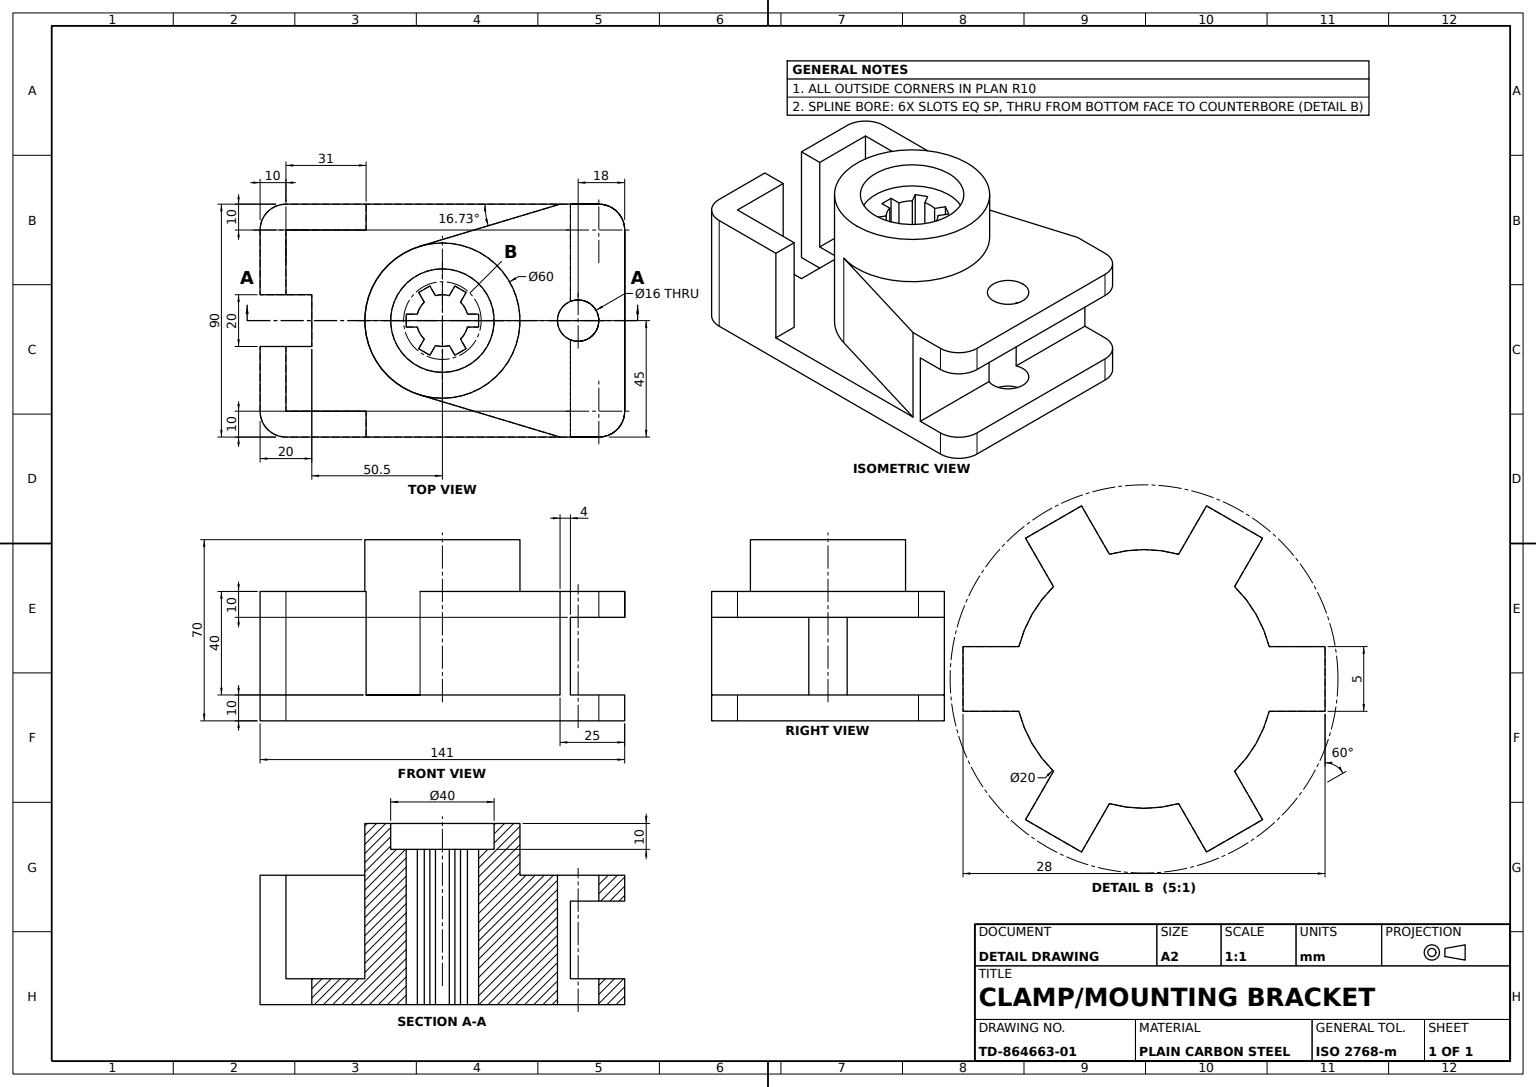
from build123d import *

# Parameters (mm, degrees)
BASE_PLATE_DEPTH     = 10
GUIDE_WALL_DEPTH     = 40
HUB_BLOCK_DEPTH      = 40
CLEVIS_START         = -10
CLEVIS_EAR_DEPTH     = 10
GUSSET_SKETCH_W      = 4
GUSSET_SKETCH_H      = 40
GUSSET_DEPTH         = 90
CROSS_HOLE_SKETCH_R  = 8
CROSS_HOLE_16_DEPTH  = 90
HUB_BOSS_SKETCH_R    = 30
HUB_BOSS_60_DEPTH    = 20
HUB_RECESS_SKETCH_R  = 20
HUB_RECESS_40_DEPTH  = 10
SPLINE_BORE_6X_DEPTH = 90


with BuildPart() as part:
    # Base Plate Sketch → Base Plate (new body)
    with BuildSketch(Plane(origin=(0, 0, 0), x_dir=(1, 0, 0), z_dir=(0, 1, 0))):
        with BuildLine():
            Line((-60.5, 45), (60.5, 45))
            ThreePointArc((60.5, 45), (67.571067812, 42.071067812), (70.5, 35))
            Line((70.5, 35), (70.5, -35))
            ThreePointArc((70.5, -35), (67.571067812, -42.071067812), (60.5, -45))
            Line((60.5, -45), (-60.5, -45))
            ThreePointArc((-60.5, -45), (-67.571067812, -42.071067812), (-70.5, -35))
            Line((-70.5, -35), (-70.5, -10))
            Line((-70.5, -10), (-50.5, -10))
            Line((-50.5, -10), (-50.5, 10))
            Line((-50.5, 10), (-70.5, 10))
            Line((-70.5, 10), (-70.5, 35))
            ThreePointArc((-70.5, 35), (-67.571067812, 42.071067812), (-60.5, 45))
        make_face()
    extrude(amount=BASE_PLATE_DEPTH)

    # Guide Wall Sketch → Guide Wall (add)
    with BuildSketch(Plane(origin=(0, 10, 0), x_dir=(1, 0, 0), z_dir=(0, 1, 0))):
        with BuildLine():
            Line((-29.5, 45), (-60.5, 45))
            ThreePointArc((-60.5, 45), (-67.571067812, 42.071067812), (-70.5, 35))
            Line((-70.5, 35), (-70.5, 10))
            Line((-70.5, 10), (-60.5, 10))
            Line((-60.5, 10), (-60.5, 35))
            Line((-60.5, 35), (-29.5, 35))
            Line((-29.5, 35), (-29.5, 45))
        make_face()
        with BuildLine():
            Line((-70.5, -10), (-70.5, -35))
            ThreePointArc((-70.5, -35), (-67.571067812, -42.071067812), (-60.5, -45))
            Line((-60.5, -45), (-29.5, -45))
            Line((-29.5, -45), (-29.5, -35))
            Line((-29.5, -35), (-60.5, -35))
            Line((-60.5, -35), (-60.5, -10))
            Line((-60.5, -10), (-70.5, -10))
        make_face()
    extrude(amount=GUIDE_WALL_DEPTH)

    # Hub Block Sketch → Hub Block (add)
    with BuildSketch(Plane(origin=(0, 10, 0), x_dir=(1, 0, 0), z_dir=(0, 1, 0))):
        with BuildLine():
            Line((45.5, -45), (45.5, 45))
            Line((45.5, 45), (-8.634596738, 28.730536702))
            ThreePointArc((-8.634596738, 28.730536702), (-30, 0), (-8.634596738, -28.730536702))
            Line((-8.634596738, -28.730536702), (45.5, -45))
        make_face()
    extrude(amount=HUB_BLOCK_DEPTH)

    # Clevis Ear Sketch → Clevis Ear (add)
    with BuildSketch(Plane(origin=(0, 50, 0), x_dir=(1, 0, 0), z_dir=(0, 1, 0)).offset(CLEVIS_START)):
        with BuildLine():
            Line((45.5, 45), (60.5, 45))
            ThreePointArc((60.5, 45), (67.571067812, 42.071067812), (70.5, 35))
            Line((70.5, 35), (70.5, -35))
            ThreePointArc((70.5, -35), (67.571067812, -42.071067812), (60.5, -45))
            Line((60.5, -45), (45.5, -45))
            Line((45.5, -45), (45.5, 45))
        make_face()
    extrude(amount=CLEVIS_EAR_DEPTH)

    # Gusset Sketch → Gusset (add)
    with BuildSketch(Plane.XY.offset(45)):
        with Locations((47.5, 30)):
            Rectangle(GUSSET_SKETCH_W, GUSSET_SKETCH_H)
    extrude(amount=-GUSSET_DEPTH)

    # Cross Hole Sketch → Cross Hole Ø16 (cut)
    with BuildSketch(Plane(origin=(0, 50, 0), x_dir=(1, 0, 0), z_dir=(0, 1, 0))):
        with Locations(Location((52.5, 0, 0), (0, 0, 270))):
            Circle(CROSS_HOLE_SKETCH_R)
    extrude(amount=-CROSS_HOLE_16_DEPTH, mode=Mode.SUBTRACT)

    # Hub Boss Sketch → Hub Boss Ø60 (add)
    with BuildSketch(Plane(origin=(0, 50, 0), x_dir=(1, 0, 0), z_dir=(0, 1, 0))):
        with Locations(Location((0, 0, 0), (0, 0, 106.727481019))):
            Circle(HUB_BOSS_SKETCH_R)
    extrude(amount=HUB_BOSS_60_DEPTH)

    # Hub Recess Sketch → Hub Recess Ø40 (cut)
    with BuildSketch(Plane(origin=(0, 70, 0), x_dir=(1, 0, 0), z_dir=(0, 1, 0))):
        with Locations(Location((0, 0, 0), (0, 0, 270))):
            Circle(HUB_RECESS_SKETCH_R)
    extrude(amount=-HUB_RECESS_40_DEPTH, mode=Mode.SUBTRACT)

    # Spline Bore Sketch → Spline Bore 6x (cut)
    with BuildSketch(Plane(origin=(0, 60, 0), x_dir=(1, 0, 0), z_dir=(0, 1, 0))):
        with BuildLine():
            Line((-3.703283788, -11.414275675), (-2.676165673, -9.635254916))
            ThreePointArc((-2.676165673, -9.635254916), (0, -10), (2.676165673, -9.635254916))
            Line((2.676165673, -9.635254916), (3.703283788, -11.414275675))
            Line((3.703283788, -11.414275675), (4.834936491, -13.374355653))
            Line((4.834936491, -13.374355653), (9.165063509, -10.874355653))
            Line((9.165063509, -10.874355653), (8.033410807, -8.914275675))
            Line((8.033410807, -8.914275675), (7.006292692, -7.135254916))
            ThreePointArc((7.006292692, -7.135254916), (8.660254038, -5), (9.682458366, -2.5))
            Line((9.682458366, -2.5), (11.736694594, -2.5))
            Line((11.736694594, -2.5), (14, -2.5))
            Line((14, -2.5), (14, 2.5))
            Line((14, 2.5), (11.736694594, 2.5))
            Line((11.736694594, 2.5), (9.682458366, 2.5))
            ThreePointArc((9.682458366, 2.5), (8.660254038, 5), (7.006292692, 7.135254916))
            Line((7.006292692, 7.135254916), (8.033410807, 8.914275675))
            Line((8.033410807, 8.914275675), (9.165063509, 10.874355653))
            Line((9.165063509, 10.874355653), (4.834936491, 13.374355653))
            Line((4.834936491, 13.374355653), (3.703283788, 11.414275675))
            Line((3.703283788, 11.414275675), (2.676165673, 9.635254916))
            ThreePointArc((2.676165673, 9.635254916), (0, 10), (-2.676165673, 9.635254916))
            Line((-2.676165673, 9.635254916), (-3.703283788, 11.414275675))
            Line((-3.703283788, 11.414275675), (-4.834936491, 13.374355653))
            Line((-4.834936491, 13.374355653), (-9.165063509, 10.874355653))
            Line((-9.165063509, 10.874355653), (-8.033410807, 8.914275675))
            Line((-8.033410807, 8.914275675), (-7.006292692, 7.135254916))
            ThreePointArc((-7.006292692, 7.135254916), (-8.660254038, 5), (-9.682458366, 2.5))
            Line((-9.682458366, 2.5), (-11.736694594, 2.5))
            Line((-11.736694594, 2.5), (-14, 2.5))
            Line((-14, 2.5), (-14, -2.5))
            Line((-14, -2.5), (-11.736694594, -2.5))
            Line((-11.736694594, -2.5), (-9.682458366, -2.5))
            ThreePointArc((-9.682458366, -2.5), (-8.660254038, -5), (-7.006292692, -7.135254916))
            Line((-7.006292692, -7.135254916), (-8.033410807, -8.914275675))
            Line((-8.033410807, -8.914275675), (-9.165063509, -10.874355653))
            Line((-9.165063509, -10.874355653), (-4.834936491, -13.374355653))
            Line((-4.834936491, -13.374355653), (-3.703283788, -11.414275675))
        make_face()
    extrude(amount=-SPLINE_BORE_6X_DEPTH, mode=Mode.SUBTRACT)


solid = part.part
